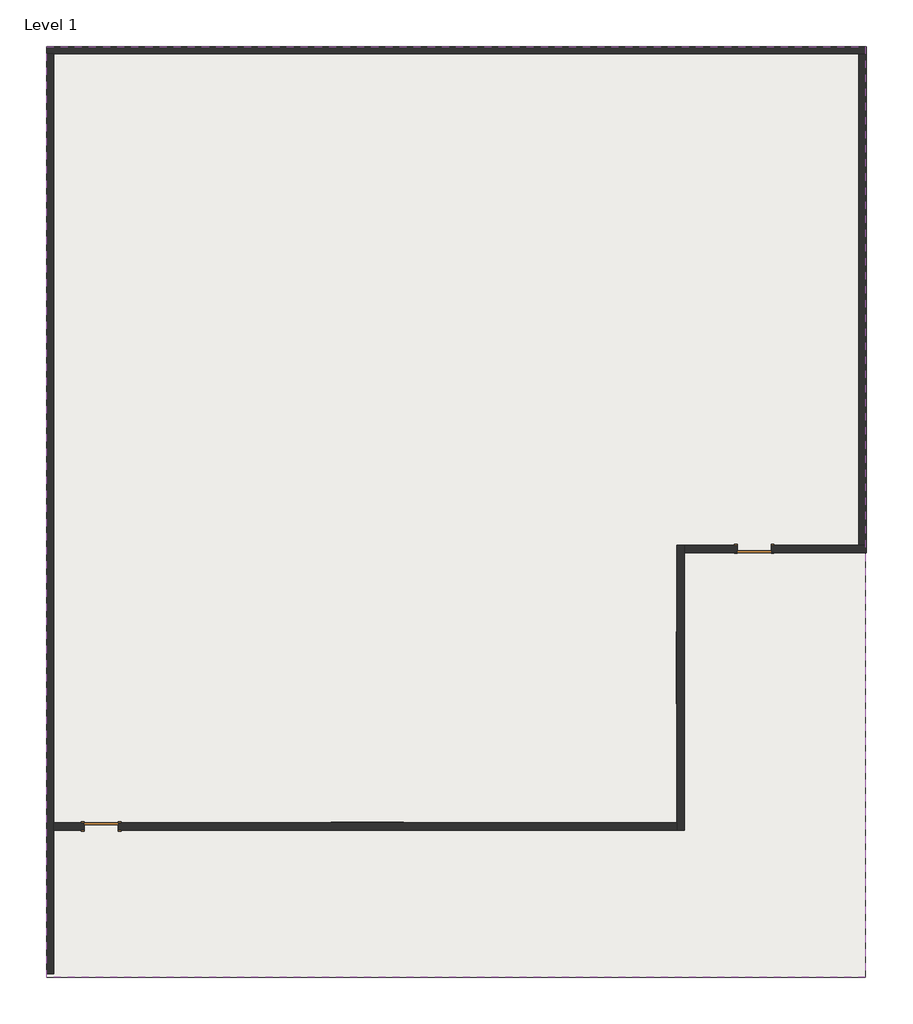
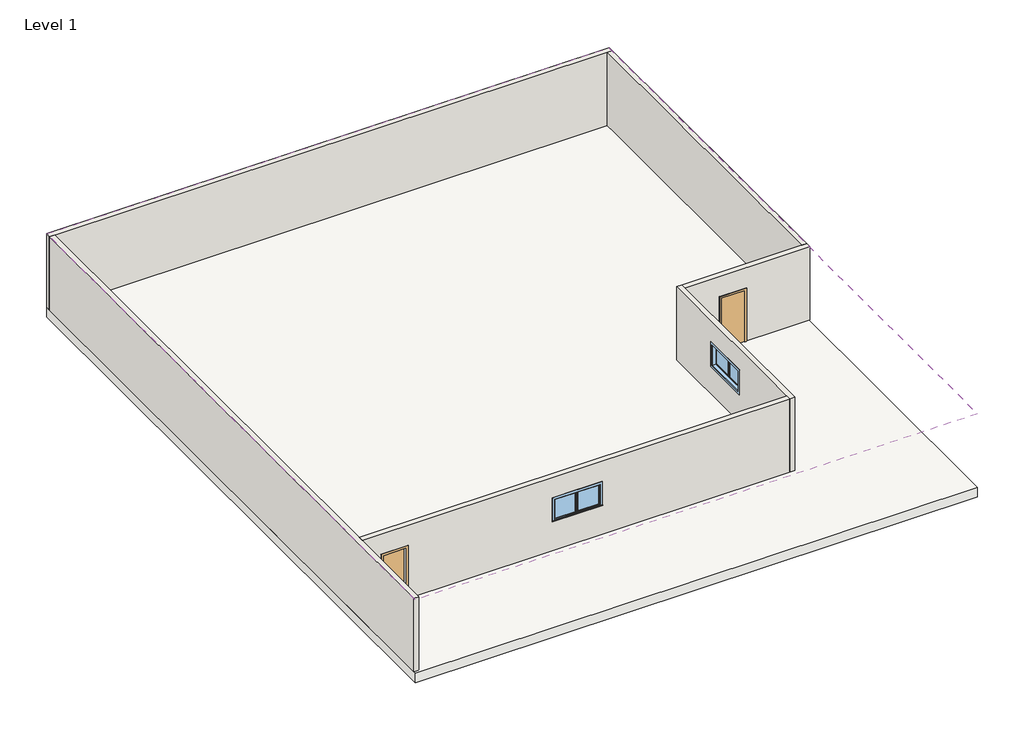
# One storey: 6 walls, 2 doors, 2 windows, 1 covering, 1 slab.
"""IFC4 building model written with IfcOpenShell, lengths in millimetres."""

from ifc_helpers import new_model, si_unit, frame, origin, place, context, project, spatial, polyline, outline, extrude, faceted_brep, transform, mapped, element, save
from components import m_single_flush_0915_x_2134mm_727434cd, m_single_flush_0915_x_2134mm_6a9e8738, window_6fce5177

model = new_model("IFC4")

# Units and contexts
model_context = context("Model", 3, world=origin())
ifc_project = project(units=[si_unit("LENGTHUNIT", "METRE", prefix="MILLI")], contexts=[model_context])

# Site, building, storey
site = spatial("IfcSite", under=ifc_project)
building = spatial("IfcBuilding", under=site)
storey = spatial("IfcBuildingStorey", under=building, Name="Level 1", Elevation=3048.0)

# Covering
placement = place(None, origin())
element("IfcCovering", 1, ObjectType="600 x 1200mm grid", at=placement, inside=storey, context=model_context, shape_type="SweptSolid", body=[
    extrude(outline(polyline([(-10207.1494882, 15306.8421936), (11835.2505118, 15306.8421936), (11835.2505118, -9734.3578064), (-10207.1494882, -9734.3578064), (-10207.1494882, 15306.8421936)])), frame((0.0, 0.0, 6096.0), z_axis=(0.0, 0.0, 1.0), x_axis=(1.0, 0.0, 0.0)), (0.0, 0.0, 1.0), 52.0),
])

# Doors
m_single_flush_0915_x_2134mm_shape = m_single_flush_0915_x_2134mm_727434cd(model_context)
element("IfcDoor", 2, ObjectType="M_Single-Flush : 0915 x 2134mm", at=placement, inside=storey, context=model_context, shape_type="MappedRepresentation", body=[
    mapped(m_single_flush_0915_x_2134mm_shape, transform((-8735.5494882, -5671.9578064, 3048.0), x_axis=(-1.0, 0.0, 0.0), y_axis=(0.0, -1.0, 0.0), z_axis=(0.0, 0.0, 1.0))),
])
m_single_flush_0915_x_2134mm_2_shape = m_single_flush_0915_x_2134mm_6a9e8738(model_context)
element("IfcDoor", 3, ObjectType="M_Single-Flush : 0915 x 2134mm", at=placement, inside=storey, context=model_context, shape_type="MappedRepresentation", body=[
    mapped(m_single_flush_0915_x_2134mm_2_shape, transform((8839.6505118, 1795.6421936, 3048.0), x_axis=(-1.0, 0.0, 0.0), y_axis=(0.0, -1.0, 0.0), z_axis=(0.0, 0.0, 1.0))),
])

# Slab
element("IfcSlab", 4, ObjectType="Generic Floor - 400mm", at=placement, inside=storey, context=model_context, shape_type="SweptSolid", body=[
    extrude(outline(polyline([(11835.2505118, 15306.8421936), (11835.2505118, -9734.3578064), (-10207.1494882, -9734.3578064), (-10207.1494882, 15306.8421936), (11835.2505118, 15306.8421936)])), frame((0.0, 0.0, 2648.0), z_axis=(0.0, 0.0, 1.0), x_axis=(1.0, 0.0, 0.0)), (0.0, 0.0, 1.0), 400.0),
])

# Walls
element("IfcWall", 5, ObjectType="Generic - 9\"", at=placement, inside=storey, context=model_context, shape_type="Brep", body=[
    faceted_brep([(-10207.1494882, 15106.8421936, 3048.0), (-10007.1494882, 15106.8421936, 3048.0), (11660.6505118, 15106.8421936, 3048.0), (11860.6505118, 15106.8421936, 3048.0), (11860.6505118, 15106.8421936, 6096.0), (11660.6505118, 15106.8421936, 6096.0), (-10007.1494882, 15106.8421936, 6096.0), (-10207.1494882, 15106.8421936, 6096.0), (-10207.1494882, 15306.8421936, 3048.0), (-10207.1494882, 15306.8421936, 6096.0), (11860.6505118, 15306.8421936, 6096.0), (11860.6505118, 15306.8421936, 3048.0)], [[[0, 1, 2, 3, 4, 5, 6, 7]], [[8, 9, 10, 11]], [[3, 2, 1, 0, 8, 11]], [[7, 6, 5, 4, 10, 9]], [[0, 7, 9, 8]], [[4, 3, 11, 10]]]),
])
element("IfcWall", 6, ObjectType="Generic - 9\"", at=placement, inside=storey, context=model_context, shape_type="Brep", body=[
    faceted_brep([(-10007.1494882, -9634.3578064, 3048.0), (-10007.1494882, -5771.9578064, 3048.0), (-10007.1494882, -5571.9578064, 3048.0), (-10007.1494882, 15106.8421936, 3048.0), (-10007.1494882, 15106.8421936, 6096.0), (-10007.1494882, -5571.9578064, 6096.0), (-10007.1494882, -5771.9578064, 6096.0), (-10007.1494882, -9634.3578064, 6096.0), (-10207.1494882, -9634.3578064, 3048.0), (-10207.1494882, -9634.3578064, 6096.0), (-10207.1494882, 15106.8421936, 6096.0), (-10207.1494882, 15106.8421936, 3048.0)], [[[0, 1, 2, 3, 4, 5, 6, 7]], [[8, 9, 10, 11]], [[3, 2, 1, 0, 8, 11]], [[7, 6, 5, 4, 10, 9]], [[0, 7, 9, 8]], [[4, 3, 11, 10]]]),
])
element("IfcWall", 7, ObjectType="Generic - 9\"", at=placement, inside=storey, context=model_context, shape_type="SweptSolid", body=[
    extrude(outline(polyline([(3048.0, -10007.1494882), (3048.0, -9193.0494882), (5182.0, -9193.0494882), (5182.0, -8278.0494882), (3048.0, -8278.0494882), (3048.0, 6758.4505118), (6096.0, 6758.4505118), (6096.0, -10007.1494882), (3048.0, -10007.1494882)]), holes=[polyline([(5181.6, -2487.1494882), (5181.6, -658.3494882), (4267.2, -658.3494882), (4267.2, -2487.1494882), (5181.6, -2487.1494882)])]), frame((0.0, -5771.9578064, 0.0), z_axis=(0.0, 1.0, 0.0), x_axis=(0.0, 0.0, 1.0)), (0.0, 0.0, 1.0), 200.0),
])
element("IfcWall", 8, ObjectType="Generic - 9\"", at=placement, inside=storey, context=model_context, shape_type="Brep", body=[
    faceted_brep([(6958.4505118, -5771.9578064, 3048.0), (6958.4505118, 1695.6421936, 3048.0), (6958.4505118, 1895.6421936, 3048.0), (6958.4505118, 1895.6421936, 6096.0), (6958.4505118, 1695.6421936, 6096.0), (6958.4505118, -5771.9578064, 6096.0), (6958.4505118, -2319.1578064, 5181.6), (6958.4505118, -490.3578064, 5181.6), (6958.4505118, -490.3578064, 4267.2), (6958.4505118, -2319.1578064, 4267.2), (6758.4505118, -5771.9578064, 3048.0), (6758.4505118, -5771.9578064, 6096.0), (6758.4505118, -5571.9578064, 6096.0), (6758.4505118, 1895.6421936, 6096.0), (6758.4505118, 1895.6421936, 3048.0), (6758.4505118, -5571.9578064, 3048.0), (6758.4505118, -2319.1578064, 5181.6), (6758.4505118, -2319.1578064, 4267.2), (6758.4505118, -490.3578064, 4267.2), (6758.4505118, -490.3578064, 5181.6)], [[[0, 1, 2, 3, 4, 5], [6, 7, 8, 9]], [[10, 11, 12, 13, 14, 15], [16, 17, 18, 19]], [[2, 1, 0, 10, 15, 14]], [[5, 4, 3, 13, 12, 11]], [[3, 2, 14, 13]], [[0, 5, 11, 10]], [[17, 16, 6, 9]], [[18, 17, 9, 8]], [[19, 18, 8, 7]], [[16, 19, 7, 6]]]),
])
element("IfcWall", 9, ObjectType="Generic - 9\"", at=placement, inside=storey, context=model_context, shape_type="Brep", body=[
    faceted_brep([(6958.4505118, 1695.6421936, 3048.0), (8382.1505118, 1695.6421936, 3048.0), (8382.1505118, 1695.6421936, 5182.0), (9297.1505118, 1695.6421936, 5182.0), (9297.1505118, 1695.6421936, 3048.0), (11860.6505118, 1695.6421936, 3048.0), (11860.6505118, 1695.6421936, 6096.0), (6958.4505118, 1695.6421936, 6096.0), (8382.1505118, 1895.6421936, 5182.0), (8382.1505118, 1895.6421936, 3048.0), (6958.4505118, 1895.6421936, 3048.0), (6958.4505118, 1895.6421936, 6096.0), (11660.6505118, 1895.6421936, 6096.0), (11860.6505118, 1895.6421936, 6096.0), (11860.6505118, 1895.6421936, 3048.0), (11660.6505118, 1895.6421936, 3048.0), (9297.1505118, 1895.6421936, 3048.0), (9297.1505118, 1895.6421936, 5182.0)], [[[0, 1, 2, 3, 4, 5, 6, 7]], [[8, 9, 10, 11, 12, 13, 14, 15, 16, 17]], [[10, 9, 1, 0]], [[16, 15, 14, 5, 4]], [[7, 6, 13, 12, 11]], [[0, 7, 11, 10]], [[6, 5, 14, 13]], [[2, 1, 9, 8]], [[3, 2, 8, 17]], [[4, 3, 17, 16]]]),
])
element("IfcWall", 10, ObjectType="Generic - 9\"", at=placement, inside=storey, context=model_context, shape_type="SweptSolid", body=[
    extrude(outline(polyline([(11860.6505118, 15106.8421936), (11860.6505118, 1895.6421936), (11660.6505118, 1895.6421936), (11660.6505118, 15106.8421936), (11860.6505118, 15106.8421936)])), frame((0.0, 0.0, 3048.0), z_axis=(0.0, 0.0, 1.0), x_axis=(1.0, 0.0, 0.0)), (0.0, 0.0, 1.0), 3048.0),
])

# Windows
window_shape = window_6fce5177(model_context)
element("IfcWindow", 11, ObjectType="Casement Dbl with Trim : 72\" x 36\"", at=placement, inside=storey, context=model_context, shape_type="MappedRepresentation", body=[
    mapped(window_shape, transform((-1572.7494882, -5652.9078064, 3048.0), x_axis=(-1.0, 0.0, 0.0), y_axis=(0.0, -1.0, 0.0), z_axis=(0.0, 0.0, 1.0))),
])
element("IfcWindow", 12, ObjectType="Casement Dbl with Trim : 72\" x 36\"", at=placement, inside=storey, context=model_context, shape_type="MappedRepresentation", body=[
    mapped(window_shape, transform((6839.4005118, -1404.7578064, 3048.0), x_axis=(0.0, -1.0, 0.0), y_axis=(1.0, 0.0, 0.0), z_axis=(0.0, 0.0, 1.0))),
])

save(model, "model.ifc")

# Revit data of these elements
# Type "600 x 1200mm grid"
#   built-in parameter 1002203 = 1 (stored number, unit not read)
#   built-in parameter 1002202 = 1 (stored number, unit not read)
#   Layers, outside or top first: 0' - 1.41732" "Default" (function 1); 0' - 0.62992" "Ceiling Tile 600 x 1200" (function 5)
# Type "M_Single-Flush : 0915 x 2134mm"
#   Type Mark = "15"
#   Thickness = 0' - 2.00787"
#   Height = 7' - 0.01575"
#   Trim Projection Ext = 0' - 0.98425"
#   Trim Projection Int = 0' - 0.98425"
#   Trim Width = 0' - 2.99213"
#   Width = 3' - 0.02362"
#   Door Material = Door - Panel
#   Frame Material = Door - Frame
#   Function = (empty or 0)
#   Wall Closure = (empty or 0)
# Type "Generic Floor - 400mm"
#   Function = 0
#   Layers, outside or top first: 1' - 3.74803" no material (function 1)
# Type "Generic - 9\""
#   Layers, outside or top first: 0' - 7.87402" no material (function 1)
# Type "Casement Dbl with Trim : 72\" x 36\""
#   Type Mark = "20"
#   Construction Type Id = "GSP4R"
#   Assembly Code = "B2020100"
#   Analytic Construction = "1/8 in Pilkington single glazing"
#   Visual Light Transmittance = 0.9
#   Solar Heat Gain Coefficient = 0.78
#   Heat Transfer Coefficient (U) = 3.6886 W/(m²·K)
#   Height = 3' - 0"
#   Default Sill Height = 4' - 0"
#   Trim Projection - Ext. = 0' - 0 1/2"
#   Trim Projection - Int. = 0' - 0 3/4"
#   Trim Width - Exterior = 0' - 3 1/2"
#   Trim Width - Interior = 0' - 3 1/2"
#   Width = 6' - 0"
#   Window Inset = 0' - 0 3/4"
#   Define Thermal Properties by = 1
#   Glass Pane Material = Glass
#   Sash Material = Sash
#   Trim Exterior Material = Trim
#   Trim Interior Material = Trim
#   Wall Closure = (empty or 0)
# Element 1 (IfcCovering, "600 x 1200mm grid")
#   Height Offset From Level = 10' - 0"
#   Phase Created = New Construction
#   Materials on its faces: "Ceiling Tile 600 x 1200", "Default"
# Elements 2, 3 (IfcDoor, "M_Single-Flush : 0915 x 2134mm")
#   Phase Created = New Construction
#   Materials on its faces: "Door - Frame", "Door - Panel"
# Element 4 (IfcSlab, "Generic Floor - 400mm")
#   Height Offset From Level = 0' - 0"
#   Phase Created = New Construction
#   Materials on its faces: "Default Roof"
# Elements 5, 6, 7, 8, 9, 10 (IfcWall, "Generic - 9\"")
#   Top Offset = 0' - 0"
#   Base Offset = 0' - 0"
#   Unconnected Height = 10' - 0"
#   wall height = 10' - 0"
#   Phase Created = New Construction
#   Base Constraint = Level 1
#   Materials on its faces: "Default Wall"
# Element 11 (IfcWindow, "Casement Dbl with Trim : 72\" x 36\"")
#   Mark = "8"
#   Phase Created = New Construction
#   Materials on its faces: "Sash", "Trim", "Glass"
# Element 12 (IfcWindow, "Casement Dbl with Trim : 72\" x 36\"")
#   Mark = "9"
#   Phase Created = New Construction
#   Materials on its faces: "Sash", "Trim", "Glass"
# Materials
#   "Default": colour RGB 80 80 80, transparency 0
#   "Ceiling Tile 600 x 1200": class "Generic", colour RGB 179 178 175, transparency 0, Description = "Acoustic ceiling tile", Cost = 0
#   "Door - Panel": class "Wood", colour RGB 114 82 51, transparency 0
#   "Door - Frame": colour RGB 153 76 43, transparency 0
#   "Glass": class "Glass", colour RGB 218 227 224, transparency 0.85, Description = "Soda Lime Glass", Cost = 0
#   "Sash": class "Wood", colour RGB 136 99 55, transparency 0
#   "Trim": class "Wood", colour RGB 224 178 126, transparency 0
#   "Default Roof": colour RGB 80 80 80, transparency 0
#   "Default Wall": colour RGB 80 80 80, transparency 0
